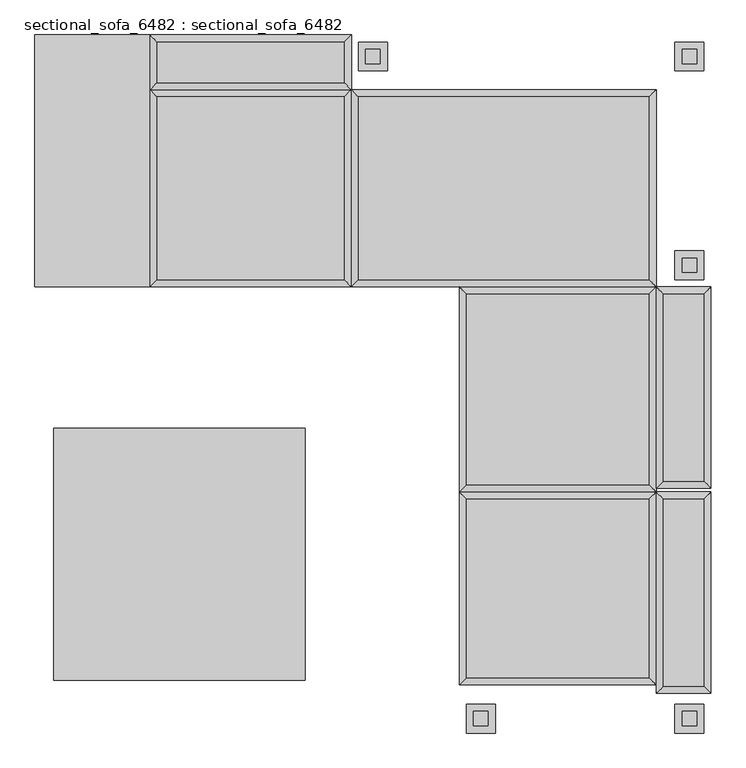
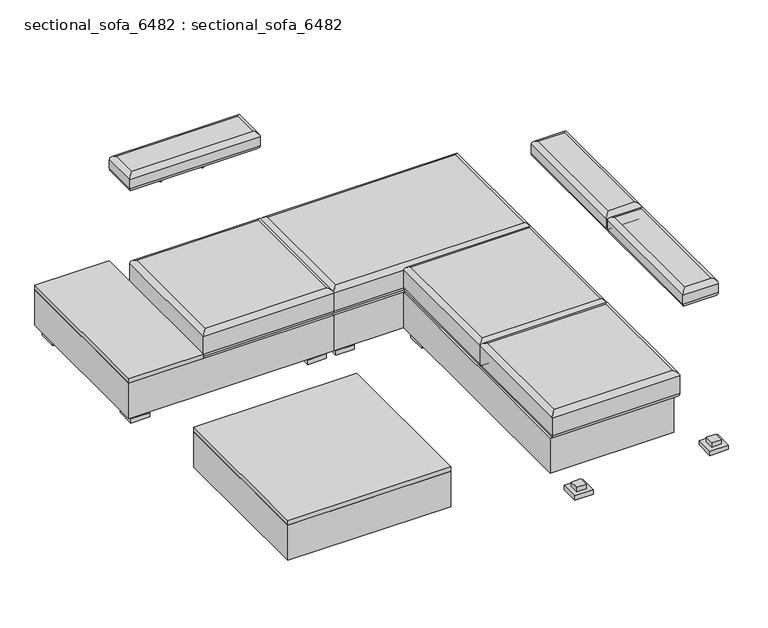
"""IFC4 building model written with IfcOpenShell, lengths in millimetres: proxy geometry, sectional_sofa_6482 : sectional_sofa_6482."""

from ifc_helpers import new_model, si_unit, point, frame, frame_2d, origin, place, context, project, spatial, polyline, circle_curve, ellipse_curve, trimmed, segment, composite_curve, outline, extrude, faceted_brep, source, transform, mapped, element, save
from ifc_brep_helpers import plane_surface, cylinder_surface, advanced_brep


def sectional_sofa_6482_sectional_sofa_6482_559db2f0(model_context):
    return source(origin(), model_context, "Body", "SolidModel", [
        extrude(outline(polyline([(-712.932438, 1291.6931081), (-712.932438, 1077.8583572), (-1.732438, 1077.8583572), (-1.732438, 402.6931081), (-1119.332438, 402.6931081), (-1119.332438, 1291.6931081), (-712.932438, 1291.6931081)])), frame((0.0, 0.0, 50.8), z_axis=(0.0, 0.0, 1.0), x_axis=(1.0, 0.0, 0.0)), (0.0, 0.0, 1.0), 203.2),
        extrude(outline(polyline([(1054.4328112, 1077.8583572), (1054.4328112, 402.6931081), (-1.732438, 402.6931081), (-1.732438, 1077.8583572), (1054.4328112, 1077.8583572)])), frame((0.0, 0.0, 50.8), z_axis=(0.0, 0.0, 1.0), x_axis=(1.0, 0.0, 0.0)), (0.0, 0.0, 1.0), 203.2),
        extrude(outline(polyline([(1054.4328112, -983.672141), (379.267562, -983.672141), (379.267562, 402.6931081), (1054.4328112, 402.6931081), (1054.4328112, -983.672141)])), frame((0.0, 0.0, 50.8), z_axis=(0.0, 0.0, 1.0), x_axis=(1.0, 0.0, 0.0)), (0.0, 0.0, 1.0), 203.2),
        faceted_brep([(-712.932438, 1291.6931081, 279.4), (-1119.332438, 1291.6931081, 279.4), (-1119.332438, 402.6931081, 279.4), (-712.932438, 402.6931081, 279.4), (-712.932438, 1098.2849958, 279.4), (-712.932438, 402.6931081, 254.0), (-1119.332438, 402.6931081, 254.0), (-1119.332438, 1291.6931081, 254.0), (-712.932438, 1291.6931081, 254.0), (-712.932438, 1098.2849958, 254.0)], [[[0, 1, 2, 3, 4]], [[5, 6, 7, 8, 9]], [[1, 0, 8, 7]], [[2, 1, 7, 6]], [[3, 2, 6, 5]], [[8, 0, 4, 3, 5, 9]]]),
        advanced_brep(
        [(404.667562, -346.6068919, 406.4), (404.667562, -977.0009907, 406.4), (1049.4594497, -977.0009907, 406.4), (1049.4594497, -346.6068919, 406.4), (404.667562, -977.0009907, 254.0), (404.667562, -346.6068919, 254.0), (1049.4594497, -346.6068919, 254.0), (1049.4594497, -977.0009907, 254.0), (1074.8594497, -321.2068919, 279.4), (1074.8594497, -321.2068919, 381.0), (1074.8594497, -1002.4009907, 381.0), (1074.8594497, -1002.4009907, 279.4), (379.267562, -321.2068919, 279.4), (379.267562, -321.2068919, 381.0), (379.267562, -1002.4009907, 279.4), (379.267562, -1002.4009907, 381.0)],
        [
            (0, 1),
            (1, 2),
            (2, 3),
            (3, 0),
            (4, 5),
            (5, 6),
            (6, 7),
            (7, 4),
            (8, 9),
            (9, 10),
            (10, 11),
            (11, 8),
            (8, 12),
            (12, 13),
            (13, 9),
            (12, 14),
            (14, 15),
            (15, 13),
            (10, 15),
            (14, 11),
            (15, 1, ellipse_curve(frame((404.667562, -977.0009907, 381.0), z_axis=(-0.7071067811865459, 0.707106781186549, 0.0), x_axis=(-0.7071067811865489, -0.7071067811865462, 0.0)), 35.9210245, 25.4)),
            (0, 13, ellipse_curve(frame((404.667562, -346.6068919, 381.0), z_axis=(-0.7071067811865489, -0.707106781186546, 0.0), x_axis=(0.707106781186546, -0.7071067811865489, 0.0)), 35.9210245, 25.4)),
            (4, 14, ellipse_curve(frame((404.667562, -977.0009907, 279.4), z_axis=(-0.7071067811865459, 0.707106781186549, 0.0), x_axis=(-0.7071067811865489, -0.7071067811865462, 0.0)), 35.9210245, 25.4)),
            (12, 5, ellipse_curve(frame((404.667562, -346.6068919, 279.4), z_axis=(-0.7071067811865489, -0.707106781186546, 0.0), x_axis=(0.707106781186546, -0.7071067811865489, 0.0)), 35.9210245, 25.4)),
            (10, 2, ellipse_curve(frame((1049.4594497, -977.0009907, 381.0), z_axis=(-0.707106781186549, -0.707106781186546, 0.0), x_axis=(0.7071067811865461, -0.7071067811865489, 0.0)), 35.9210245, 25.4)),
            (7, 11, ellipse_curve(frame((1049.4594497, -977.0009907, 279.4), z_axis=(-0.707106781186549, -0.707106781186546, 0.0), x_axis=(0.7071067811865461, -0.7071067811865489, 0.0)), 35.9210245, 25.4)),
            (9, 3, ellipse_curve(frame((1049.4594497, -346.6068919, 381.0), z_axis=(0.7071067811865461, -0.7071067811865489, 0.0), x_axis=(0.7071067811865489, 0.7071067811865461, 0.0)), 35.9210245, 25.4)),
            (6, 8, ellipse_curve(frame((1049.4594497, -346.6068919, 279.4), z_axis=(0.7071067811865461, -0.7071067811865489, 0.0), x_axis=(0.7071067811865489, 0.7071067811865461, 0.0)), 35.9210245, 25.4)),
        ],
        [
            plane_surface(frame((1074.8594497, -333.9068919, 406.4), z_axis=(0.0, 0.0, 1.0), x_axis=(0.0, 1.0, 0.0))),
            plane_surface(frame((1074.8594497, -333.9068919, 254.0), z_axis=(0.0, 0.0, -1.0), x_axis=(0.0, -1.0, 0.0))),
            plane_surface(frame((1074.8594497, -1002.4009907, 406.4), z_axis=(1.0, 0.0, 0.0), x_axis=(0.0, 0.0, -1.0))),
            plane_surface(frame((1074.8594497, -321.2068919, 406.4), z_axis=(0.0, 1.0, 0.0), x_axis=(0.0, 0.0, -1.0))),
            plane_surface(frame((379.267562, -321.2068919, 406.4), z_axis=(-1.0, 0.0, 0.0), x_axis=(0.0, 0.0, -1.0))),
            plane_surface(frame((379.267562, -1002.4009907, 406.4), z_axis=(0.0, -1.0, 0.0), x_axis=(0.0, 0.0, -1.0))),
            cylinder_surface(frame((404.667562, -321.2068919, 381.0), z_axis=(0.0, -1.0, 0.0), x_axis=(1.0, 0.0, 0.0)), 25.4),
            cylinder_surface(frame((404.667562, -321.2068919, 279.4), z_axis=(0.0, -1.0, 0.0), x_axis=(1.0, 0.0, 0.0)), 25.4),
            cylinder_surface(frame((379.267562, -977.0009907, 381.0), z_axis=(1.0, 0.0, 0.0), x_axis=(0.0, 1.0, 0.0)), 25.4),
            cylinder_surface(frame((379.267562, -977.0009907, 279.4), z_axis=(1.0, 0.0, 0.0), x_axis=(0.0, 1.0, 0.0)), 25.4),
            cylinder_surface(frame((1049.4594497, -1002.4009907, 381.0), z_axis=(0.0, 1.0, 0.0), x_axis=(-1.0, 0.0, 0.0)), 25.4),
            cylinder_surface(frame((1049.4594497, -1002.4009907, 279.4), z_axis=(0.0, 1.0, 0.0), x_axis=(-1.0, 0.0, 0.0)), 25.4),
            cylinder_surface(frame((1074.8594497, -346.6068919, 381.0), z_axis=(-1.0, 0.0, 0.0), x_axis=(0.0, -1.0, 0.0)), 25.4),
            cylinder_surface(frame((1074.8594497, -346.6068919, 279.4), z_axis=(-1.0, 0.0, 0.0), x_axis=(0.0, -1.0, 0.0)), 25.4),
        ],
        [
            (0, [[1, 2, 3, 4]]),
            (1, [[5, 6, 7, 8]]),
            (2, [[9, 10, 11, 12]]),
            (3, [[-9, 13, 14, 15]]),
            (4, [[-14, 16, 17, 18]]),
            (5, [[-11, 19, -17, 20]]),
            (6, [[21, -1, 22, -18]]),
            (7, [[23, -16, 24, -5]]),
            (8, [[-21, -19, 25, -2]]),
            (9, [[-23, -8, 26, -20]]),
            (10, [[-25, -10, 27, -3]]),
            (11, [[-26, -7, 28, -12]]),
            (12, [[-22, -4, -27, -15]]),
            (13, [[-24, -13, -28, -6]]),
        ],
    ),
        faceted_brep([(-992.332438, 1164.6931081, 25.4), (-992.332438, 1266.2931081, 25.4), (-1093.932438, 1266.2931081, 25.4), (-1093.932438, 1164.6931081, 25.4), (-1017.732438, 1240.8931081, 25.4), (-1017.732438, 1190.0931081, 25.4), (-1068.532438, 1190.0931081, 25.4), (-1068.532438, 1240.8931081, 25.4), (-992.332438, 1164.6931081, 0.0), (-1093.932438, 1164.6931081, 0.0), (-1093.932438, 1266.2931081, 0.0), (-992.332438, 1266.2931081, 0.0), (-1017.732438, 1190.0931081, 50.8), (-1017.732438, 1240.8931081, 50.8), (-1068.532438, 1240.8931081, 50.8), (-1068.532438, 1190.0931081, 50.8)], [[[0, 1, 2, 3], [4, 5, 6, 7]], [[8, 9, 10, 11]], [[1, 0, 8, 11]], [[2, 1, 11, 10]], [[3, 2, 10, 9]], [[0, 3, 9, 8]], [[12, 13, 14, 15]], [[13, 12, 5, 4]], [[14, 13, 4, 7]], [[15, 14, 7, 6]], [[12, 15, 6, 5]]]),
        faceted_brep([(-992.332438, 428.0931081, 25.4), (-992.332438, 529.6931081, 25.4), (-1093.932438, 529.6931081, 25.4), (-1093.932438, 428.0931081, 25.4), (-1017.732438, 504.2931081, 25.4), (-1017.732438, 453.4931081, 25.4), (-1068.532438, 453.4931081, 25.4), (-1068.532438, 504.2931081, 25.4), (-992.332438, 428.0931081, 0.0), (-1093.932438, 428.0931081, 0.0), (-1093.932438, 529.6931081, 0.0), (-992.332438, 529.6931081, 0.0), (-1017.732438, 453.4931081, 50.8), (-1017.732438, 504.2931081, 50.8), (-1068.532438, 504.2931081, 50.8), (-1068.532438, 453.4931081, 50.8)], [[[0, 1, 2, 3], [4, 5, 6, 7]], [[8, 9, 10, 11]], [[1, 0, 8, 11]], [[2, 1, 11, 10]], [[3, 2, 10, 9]], [[0, 3, 9, 8]], [[12, 13, 14, 15]], [[13, 12, 5, 4]], [[14, 13, 4, 7]], [[15, 14, 7, 6]], [[12, 15, 6, 5]]]),
        faceted_brep([(-27.132438, 1164.6931081, 25.4), (-27.132438, 1266.2931081, 25.4), (-128.732438, 1266.2931081, 25.4), (-128.732438, 1164.6931081, 25.4), (-52.532438, 1240.8931081, 25.4), (-52.532438, 1190.0931081, 25.4), (-103.332438, 1190.0931081, 25.4), (-103.332438, 1240.8931081, 25.4), (-27.132438, 1164.6931081, 0.0), (-128.732438, 1164.6931081, 0.0), (-128.732438, 1266.2931081, 0.0), (-27.132438, 1266.2931081, 0.0), (-52.532438, 1190.0931081, 50.8), (-52.532438, 1240.8931081, 50.8), (-103.332438, 1240.8931081, 50.8), (-103.332438, 1190.0931081, 50.8)], [[[0, 1, 2, 3], [4, 5, 6, 7]], [[8, 9, 10, 11]], [[1, 0, 8, 11]], [[2, 1, 11, 10]], [[3, 2, 10, 9]], [[0, 3, 9, 8]], [[12, 13, 14, 15]], [[13, 12, 5, 4]], [[14, 13, 4, 7]], [[15, 14, 7, 6]], [[12, 15, 6, 5]]]),
        faceted_brep([(23.667562, 1164.6931081, 25.4), (125.267562, 1164.6931081, 25.4), (125.267562, 1266.2931081, 25.4), (23.667562, 1266.2931081, 25.4), (99.867562, 1190.0931081, 25.4), (49.067562, 1190.0931081, 25.4), (49.067562, 1240.8931081, 25.4), (99.867562, 1240.8931081, 25.4), (23.667562, 1164.6931081, 0.0), (23.667562, 1266.2931081, 0.0), (125.267562, 1266.2931081, 0.0), (125.267562, 1164.6931081, 0.0), (49.067562, 1190.0931081, 50.8), (99.867562, 1190.0931081, 50.8), (99.867562, 1240.8931081, 50.8), (49.067562, 1240.8931081, 50.8)], [[[0, 1, 2, 3], [4, 5, 6, 7]], [[8, 9, 10, 11]], [[1, 0, 8, 11]], [[2, 1, 11, 10]], [[3, 2, 10, 9]], [[0, 3, 9, 8]], [[12, 13, 14, 15]], [[13, 12, 5, 4]], [[14, 13, 4, 7]], [[15, 14, 7, 6]], [[12, 15, 6, 5]]]),
        faceted_brep([(-27.132438, 428.0931081, 25.4), (-27.132438, 529.6931081, 25.4), (-128.732438, 529.6931081, 25.4), (-128.732438, 428.0931081, 25.4), (-52.532438, 504.2931081, 25.4), (-52.532438, 453.4931081, 25.4), (-103.332438, 453.4931081, 25.4), (-103.332438, 504.2931081, 25.4), (-27.132438, 428.0931081, 0.0), (-128.732438, 428.0931081, 0.0), (-128.732438, 529.6931081, 0.0), (-27.132438, 529.6931081, 0.0), (-52.532438, 453.4931081, 50.8), (-52.532438, 504.2931081, 50.8), (-103.332438, 504.2931081, 50.8), (-103.332438, 453.4931081, 50.8)], [[[0, 1, 2, 3], [4, 5, 6, 7]], [[8, 9, 10, 11]], [[1, 0, 8, 11]], [[2, 1, 11, 10]], [[3, 2, 10, 9]], [[0, 3, 9, 8]], [[12, 13, 14, 15]], [[13, 12, 5, 4]], [[14, 13, 4, 7]], [[15, 14, 7, 6]], [[12, 15, 6, 5]]]),
        faceted_brep([(23.667562, 428.0931081, 25.4), (125.267562, 428.0931081, 25.4), (125.267562, 529.6931081, 25.4), (23.667562, 529.6931081, 25.4), (99.867562, 453.4931081, 25.4), (49.067562, 453.4931081, 25.4), (49.067562, 504.2931081, 25.4), (99.867562, 504.2931081, 25.4), (23.667562, 428.0931081, 0.0), (23.667562, 529.6931081, 0.0), (125.267562, 529.6931081, 0.0), (125.267562, 428.0931081, 0.0), (49.067562, 453.4931081, 50.8), (99.867562, 453.4931081, 50.8), (99.867562, 504.2931081, 50.8), (49.067562, 504.2931081, 50.8)], [[[0, 1, 2, 3], [4, 5, 6, 7]], [[8, 9, 10, 11]], [[1, 0, 8, 11]], [[2, 1, 11, 10]], [[3, 2, 10, 9]], [[0, 3, 9, 8]], [[12, 13, 14, 15]], [[13, 12, 5, 4]], [[14, 13, 4, 7]], [[15, 14, 7, 6]], [[12, 15, 6, 5]]]),
        faceted_brep([(1242.867562, 1164.6931081, 25.4), (1242.867562, 1266.2931081, 25.4), (1141.267562, 1266.2931081, 25.4), (1141.267562, 1164.6931081, 25.4), (1217.467562, 1240.8931081, 25.4), (1217.467562, 1190.0931081, 25.4), (1166.667562, 1190.0931081, 25.4), (1166.667562, 1240.8931081, 25.4), (1242.867562, 1164.6931081, 0.0), (1141.267562, 1164.6931081, 0.0), (1141.267562, 1266.2931081, 0.0), (1242.867562, 1266.2931081, 0.0), (1217.467562, 1190.0931081, 50.8), (1217.467562, 1240.8931081, 50.8), (1166.667562, 1240.8931081, 50.8), (1166.667562, 1190.0931081, 50.8)], [[[0, 1, 2, 3], [4, 5, 6, 7]], [[8, 9, 10, 11]], [[1, 0, 8, 11]], [[2, 1, 11, 10]], [[3, 2, 10, 9]], [[0, 3, 9, 8]], [[12, 13, 14, 15]], [[13, 12, 5, 4]], [[14, 13, 4, 7]], [[15, 14, 7, 6]], [[12, 15, 6, 5]]]),
        faceted_brep([(506.267562, 377.2931081, 25.4), (404.667562, 377.2931081, 25.4), (404.667562, 275.6931081, 25.4), (506.267562, 275.6931081, 25.4), (430.067562, 351.8931081, 25.4), (480.867562, 351.8931081, 25.4), (480.867562, 301.0931081, 25.4), (430.067562, 301.0931081, 25.4), (506.267562, 377.2931081, 0.0), (506.267562, 275.6931081, 0.0), (404.667562, 275.6931081, 0.0), (404.667562, 377.2931081, 0.0), (480.867562, 351.8931081, 50.8), (430.067562, 351.8931081, 50.8), (430.067562, 301.0931081, 50.8), (480.867562, 301.0931081, 50.8)], [[[0, 1, 2, 3], [4, 5, 6, 7]], [[8, 9, 10, 11]], [[1, 0, 8, 11]], [[2, 1, 11, 10]], [[3, 2, 10, 9]], [[0, 3, 9, 8]], [[12, 13, 14, 15]], [[13, 12, 5, 4]], [[14, 13, 4, 7]], [[15, 14, 7, 6]], [[12, 15, 6, 5]]]),
        faceted_brep([(1242.867562, 428.0931081, 25.4), (1242.867562, 529.6931081, 25.4), (1141.267562, 529.6931081, 25.4), (1141.267562, 428.0931081, 25.4), (1217.467562, 504.2931081, 25.4), (1217.467562, 453.4931081, 25.4), (1166.667562, 453.4931081, 25.4), (1166.667562, 504.2931081, 25.4), (1242.867562, 428.0931081, 0.0), (1141.267562, 428.0931081, 0.0), (1141.267562, 529.6931081, 0.0), (1242.867562, 529.6931081, 0.0), (1217.467562, 453.4931081, 50.8), (1217.467562, 504.2931081, 50.8), (1166.667562, 504.2931081, 50.8), (1166.667562, 453.4931081, 50.8)], [[[0, 1, 2, 3], [4, 5, 6, 7]], [[8, 9, 10, 11]], [[1, 0, 8, 11]], [[2, 1, 11, 10]], [[3, 2, 10, 9]], [[0, 3, 9, 8]], [[12, 13, 14, 15]], [[13, 12, 5, 4]], [[14, 13, 4, 7]], [[15, 14, 7, 6]], [[12, 15, 6, 5]]]),
        faceted_brep([(1242.867562, 377.2931081, 25.4), (1141.267562, 377.2931081, 25.4), (1141.267562, 275.6931081, 25.4), (1242.867562, 275.6931081, 25.4), (1166.667562, 351.8931081, 25.4), (1217.467562, 351.8931081, 25.4), (1217.467562, 301.0931081, 25.4), (1166.667562, 301.0931081, 25.4), (1242.867562, 377.2931081, 0.0), (1242.867562, 275.6931081, 0.0), (1141.267562, 275.6931081, 0.0), (1141.267562, 377.2931081, 0.0), (1217.467562, 351.8931081, 50.8), (1166.667562, 351.8931081, 50.8), (1166.667562, 301.0931081, 50.8), (1217.467562, 301.0931081, 50.8)], [[[0, 1, 2, 3], [4, 5, 6, 7]], [[8, 9, 10, 11]], [[1, 0, 8, 11]], [[2, 1, 11, 10]], [[3, 2, 10, 9]], [[0, 3, 9, 8]], [[12, 13, 14, 15]], [[13, 12, 5, 4]], [[14, 13, 4, 7]], [[15, 14, 7, 6]], [[12, 15, 6, 5]]]),
        faceted_brep([(506.267562, -1172.1068919, 25.4), (506.267562, -1070.5068919, 25.4), (404.667562, -1070.5068919, 25.4), (404.667562, -1172.1068919, 25.4), (480.867562, -1095.9068919, 25.4), (480.867562, -1146.7068919, 25.4), (430.067562, -1146.7068919, 25.4), (430.067562, -1095.9068919, 25.4), (506.267562, -1172.1068919, 0.0), (404.667562, -1172.1068919, 0.0), (404.667562, -1070.5068919, 0.0), (506.267562, -1070.5068919, 0.0), (480.867562, -1146.7068919, 50.8), (480.867562, -1095.9068919, 50.8), (430.067562, -1095.9068919, 50.8), (430.067562, -1146.7068919, 50.8)], [[[0, 1, 2, 3], [4, 5, 6, 7]], [[8, 9, 10, 11]], [[1, 0, 8, 11]], [[2, 1, 11, 10]], [[3, 2, 10, 9]], [[0, 3, 9, 8]], [[12, 13, 14, 15]], [[13, 12, 5, 4]], [[14, 13, 4, 7]], [[15, 14, 7, 6]], [[12, 15, 6, 5]]]),
        faceted_brep([(1242.867562, -1172.1068919, 25.4), (1242.867562, -1070.5068919, 25.4), (1141.267562, -1070.5068919, 25.4), (1141.267562, -1172.1068919, 25.4), (1217.467562, -1095.9068919, 25.4), (1217.467562, -1146.7068919, 25.4), (1166.667562, -1146.7068919, 25.4), (1166.667562, -1095.9068919, 25.4), (1242.867562, -1172.1068919, 0.0), (1141.267562, -1172.1068919, 0.0), (1141.267562, -1070.5068919, 0.0), (1242.867562, -1070.5068919, 0.0), (1217.467562, -1146.7068919, 50.8), (1217.467562, -1095.9068919, 50.8), (1166.667562, -1095.9068919, 50.8), (1166.667562, -1146.7068919, 50.8)], [[[0, 1, 2, 3], [4, 5, 6, 7]], [[8, 9, 10, 11]], [[1, 0, 8, 11]], [[2, 1, 11, 10]], [[3, 2, 10, 9]], [[0, 3, 9, 8]], [[12, 13, 14, 15]], [[13, 12, 5, 4]], [[14, 13, 4, 7]], [[15, 14, 7, 6]], [[12, 15, 6, 5]]]),
        extrude(outline(composite_curve([segment(trimmed(circle_curve(frame_2d((-482.8859111, 1206.7842798)), 6.35), [point((-489.2359111, 1206.7842798))], [point((-476.5359111, 1206.7842798))], False, "CARTESIAN"), True, "CONTINUOUS"), segment(trimmed(circle_curve(frame_2d((-482.8859111, 1206.7842798)), 6.35), [point((-476.5359111, 1206.7842798))], [point((-489.2359111, 1206.7842798))], False, "CARTESIAN"), True, "CONTINUOUS")], self_intersect=False)), frame((0.0, 0.0, 711.2), z_axis=(0.0, 0.0, 1.0), x_axis=(1.0, 0.0, 0.0)), (0.0, 0.0, 1.0), 76.2),
        extrude(outline(composite_curve([segment(trimmed(circle_curve(frame_2d((-254.2859111, 1206.7842798)), 6.35), [point((-260.6359111, 1206.7842798))], [point((-247.9359111, 1206.7842798))], False, "CARTESIAN"), True, "CONTINUOUS"), segment(trimmed(circle_curve(frame_2d((-254.2859111, 1206.7842798)), 6.35), [point((-247.9359111, 1206.7842798))], [point((-260.6359111, 1206.7842798))], False, "CARTESIAN"), True, "CONTINUOUS")], self_intersect=False)), frame((0.0, 0.0, 711.2), z_axis=(0.0, 0.0, 1.0), x_axis=(1.0, 0.0, 0.0)), (0.0, 0.0, 1.0), 76.2),
        extrude(outline(composite_curve([segment(trimmed(circle_curve(frame_2d((1173.6454882, 148.0415505)), 6.35), [point((1173.6454882, 154.3915505))], [point((1173.6454882, 141.6915505))], False, "CARTESIAN"), True, "CONTINUOUS"), segment(trimmed(circle_curve(frame_2d((1173.6454882, 148.0415505)), 6.35), [point((1173.6454882, 141.6915505))], [point((1173.6454882, 154.3915505))], False, "CARTESIAN"), True, "CONTINUOUS")], self_intersect=False)), frame((0.0, 0.0, 711.2), z_axis=(0.0, 0.0, 1.0), x_axis=(1.0, 0.0, 0.0)), (0.0, 0.0, 1.0), 76.2),
        extrude(outline(composite_curve([segment(trimmed(circle_curve(frame_2d((1173.6454882, -80.5584495)), 6.35), [point((1173.6454882, -74.2084495))], [point((1173.6454882, -86.9084495))], False, "CARTESIAN"), True, "CONTINUOUS"), segment(trimmed(circle_curve(frame_2d((1173.6454882, -80.5584495)), 6.35), [point((1173.6454882, -86.9084495))], [point((1173.6454882, -74.2084495))], False, "CARTESIAN"), True, "CONTINUOUS")], self_intersect=False)), frame((0.0, 0.0, 711.2), z_axis=(0.0, 0.0, 1.0), x_axis=(1.0, 0.0, 0.0)), (0.0, 0.0, 1.0), 76.2),
        extrude(outline(composite_curve([segment(trimmed(circle_curve(frame_2d((1173.6454882, -563.1584495)), 6.35), [point((1173.6454882, -556.8084495))], [point((1173.6454882, -569.5084495))], False, "CARTESIAN"), True, "CONTINUOUS"), segment(trimmed(circle_curve(frame_2d((1173.6454882, -563.1584495)), 6.35), [point((1173.6454882, -569.5084495))], [point((1173.6454882, -556.8084495))], False, "CARTESIAN"), True, "CONTINUOUS")], self_intersect=False)), frame((0.0, 0.0, 711.2), z_axis=(0.0, 0.0, 1.0), x_axis=(1.0, 0.0, 0.0)), (0.0, 0.0, 1.0), 76.2),
        extrude(outline(composite_curve([segment(trimmed(circle_curve(frame_2d((1173.6454882, -791.7584495)), 6.35), [point((1173.6454882, -785.4084495))], [point((1173.6454882, -798.1084495))], False, "CARTESIAN"), True, "CONTINUOUS"), segment(trimmed(circle_curve(frame_2d((1173.6454882, -791.7584495)), 6.35), [point((1173.6454882, -798.1084495))], [point((1173.6454882, -785.4084495))], False, "CARTESIAN"), True, "CONTINUOUS")], self_intersect=False)), frame((0.0, 0.0, 711.2), z_axis=(0.0, 0.0, 1.0), x_axis=(1.0, 0.0, 0.0)), (0.0, 0.0, 1.0), 76.2),
        advanced_brep(
        [(-687.532438, 1123.6849958, 889.0), (-27.132438, 1123.6849958, 889.0), (-27.132438, 1266.2931081, 889.0), (-687.532438, 1266.2931081, 889.0), (-27.132438, 1123.6849958, 787.4), (-687.532438, 1123.6849958, 787.4), (-687.532438, 1266.2931081, 787.4), (-27.132438, 1266.2931081, 787.4), (-1.732438, 1291.6931081, 863.6), (-1.732438, 1291.6931081, 812.8), (-712.932438, 1291.6931081, 812.8), (-712.932438, 1291.6931081, 863.6), (-712.932438, 1098.2849958, 812.8), (-712.932438, 1098.2849958, 863.6), (-1.732438, 1098.2849958, 812.8), (-1.732438, 1098.2849958, 863.6)],
        [
            (0, 1),
            (1, 2),
            (2, 3),
            (3, 0),
            (4, 5),
            (5, 6),
            (6, 7),
            (7, 4),
            (8, 9),
            (9, 10),
            (10, 11),
            (11, 8),
            (10, 12),
            (12, 13),
            (13, 11),
            (12, 14),
            (14, 15),
            (15, 13),
            (8, 15),
            (14, 9),
            (15, 1, ellipse_curve(frame((-27.132438, 1123.6849958, 863.6), z_axis=(-0.7071067811865475, -0.7071067811865475, 0.0), x_axis=(0.7071067811865476, -0.7071067811865474, 0.0)), 35.9210245, 25.4)),
            (0, 13, ellipse_curve(frame((-687.532438, 1123.6849958, 863.6), z_axis=(0.7071067811865475, -0.7071067811865475, 0.0), x_axis=(0.7071067811865476, 0.7071067811865474, 0.0)), 35.9210245, 25.4)),
            (4, 14, ellipse_curve(frame((-27.132438, 1123.6849958, 812.8), z_axis=(-0.7071067811865475, -0.7071067811865475, 0.0), x_axis=(0.7071067811865476, -0.7071067811865474, 0.0)), 35.9210245, 25.4)),
            (12, 5, ellipse_curve(frame((-687.532438, 1123.6849958, 812.8), z_axis=(0.7071067811865475, -0.7071067811865475, 0.0), x_axis=(0.7071067811865476, 0.7071067811865474, 0.0)), 35.9210245, 25.4)),
            (8, 2, ellipse_curve(frame((-27.132438, 1266.2931081, 863.6), z_axis=(0.7071067811865475, -0.7071067811865475, 0.0), x_axis=(0.7071067811865474, 0.7071067811865476, 0.0)), 35.9210245, 25.4)),
            (7, 9, ellipse_curve(frame((-27.132438, 1266.2931081, 812.8), z_axis=(0.7071067811865475, -0.7071067811865475, 0.0), x_axis=(0.7071067811865474, 0.7071067811865476, 0.0)), 35.9210245, 25.4)),
            (11, 3, ellipse_curve(frame((-687.532438, 1266.2931081, 863.6), z_axis=(0.7071067811865475, 0.7071067811865475, 0.0), x_axis=(-0.7071067811865476, 0.7071067811865474, 0.0)), 35.9210245, 25.4)),
            (6, 10, ellipse_curve(frame((-687.532438, 1266.2931081, 812.8), z_axis=(0.7071067811865475, 0.7071067811865475, 0.0), x_axis=(-0.7071067811865476, 0.7071067811865474, 0.0)), 35.9210245, 25.4)),
        ],
        [
            plane_surface(frame((-712.932438, 1291.6931081, 889.0), z_axis=(0.0, 0.0, 1.0), x_axis=(-1.0, 0.0, 0.0))),
            plane_surface(frame((-712.932438, 1291.6931081, 787.4), z_axis=(0.0, 0.0, -1.0), x_axis=(1.0, 0.0, 0.0))),
            plane_surface(frame((-1.732438, 1291.6931081, 889.0), z_axis=(0.0, 1.0, 0.0), x_axis=(0.0, 0.0, -1.0))),
            plane_surface(frame((-712.932438, 1291.6931081, 889.0), z_axis=(-1.0, 0.0, 0.0), x_axis=(0.0, 0.0, -1.0))),
            plane_surface(frame((-712.932438, 1098.2849958, 889.0), z_axis=(0.0, -1.0, 0.0), x_axis=(0.0, 0.0, -1.0))),
            plane_surface(frame((-1.732438, 1098.2849958, 889.0), z_axis=(1.0, 0.0, 0.0), x_axis=(0.0, 0.0, -1.0))),
            cylinder_surface(frame((-712.932438, 1123.6849958, 863.6), z_axis=(1.0, 0.0, 0.0), x_axis=(0.0, 1.0, 0.0)), 25.4),
            cylinder_surface(frame((-712.932438, 1123.6849958, 812.8), z_axis=(1.0, 0.0, 0.0), x_axis=(0.0, 1.0, 0.0)), 25.4),
            cylinder_surface(frame((-27.132438, 1098.2849958, 863.6), z_axis=(0.0, 1.0, 0.0), x_axis=(-1.0, 0.0, 0.0)), 25.4),
            cylinder_surface(frame((-27.132438, 1098.2849958, 812.8), z_axis=(0.0, 1.0, 0.0), x_axis=(-1.0, 0.0, 0.0)), 25.4),
            cylinder_surface(frame((-1.732438, 1266.2931081, 863.6), z_axis=(-1.0, 0.0, 0.0), x_axis=(0.0, -1.0, 0.0)), 25.4),
            cylinder_surface(frame((-1.732438, 1266.2931081, 812.8), z_axis=(-1.0, 0.0, 0.0), x_axis=(0.0, -1.0, 0.0)), 25.4),
            cylinder_surface(frame((-687.532438, 1291.6931081, 863.6), z_axis=(0.0, -1.0, 0.0), x_axis=(1.0, 0.0, 0.0)), 25.4),
            cylinder_surface(frame((-687.532438, 1291.6931081, 812.8), z_axis=(0.0, -1.0, 0.0), x_axis=(1.0, 0.0, 0.0)), 25.4),
        ],
        [
            (0, [[1, 2, 3, 4]]),
            (1, [[5, 6, 7, 8]]),
            (2, [[9, 10, 11, 12]]),
            (3, [[-11, 13, 14, 15]]),
            (4, [[-14, 16, 17, 18]]),
            (5, [[-9, 19, -17, 20]]),
            (6, [[21, -1, 22, -18]]),
            (7, [[23, -16, 24, -5]]),
            (8, [[-21, -19, 25, -2]]),
            (9, [[-23, -8, 26, -20]]),
            (10, [[-25, -12, 27, -3]]),
            (11, [[-26, -7, 28, -10]]),
            (12, [[-22, -4, -27, -15]]),
            (13, [[-24, -13, -28, -6]]),
        ],
    ),
        advanced_brep(
        [(1100.2594497, 377.2931081, 889.0), (1100.2594497, -283.1068919, 889.0), (1242.867562, -283.1068919, 889.0), (1242.867562, 377.2931081, 889.0), (1100.2594497, -283.1068919, 787.4), (1100.2594497, 377.2931081, 787.4), (1242.867562, 377.2931081, 787.4), (1242.867562, -283.1068919, 787.4), (1268.267562, -308.5068919, 863.6), (1268.267562, -308.5068919, 812.8), (1268.267562, 402.6931081, 812.8), (1268.267562, 402.6931081, 863.6), (1074.8594497, 402.6931081, 812.8), (1074.8594497, 402.6931081, 863.6), (1074.8594497, -308.5068919, 812.8), (1074.8594497, -308.5068919, 863.6)],
        [
            (0, 1),
            (1, 2),
            (2, 3),
            (3, 0),
            (4, 5),
            (5, 6),
            (6, 7),
            (7, 4),
            (8, 9),
            (9, 10),
            (10, 11),
            (11, 8),
            (10, 12),
            (12, 13),
            (13, 11),
            (12, 14),
            (14, 15),
            (15, 13),
            (8, 15),
            (14, 9),
            (15, 1, ellipse_curve(frame((1100.2594497, -283.1068919, 863.6), z_axis=(-0.7071067811865487, 0.7071067811865462, 0.0), x_axis=(-0.7071067811865462, -0.7071067811865488, 0.0)), 35.9210245, 25.4)),
            (0, 13, ellipse_curve(frame((1100.2594497, 377.2931081, 863.6), z_axis=(-0.7071067811865461, -0.7071067811865489, 0.0), x_axis=(0.7071067811865489, -0.7071067811865461, 0.0)), 35.9210245, 25.4)),
            (4, 14, ellipse_curve(frame((1100.2594497, -283.1068919, 812.8), z_axis=(-0.7071067811865487, 0.7071067811865462, 0.0), x_axis=(-0.7071067811865462, -0.7071067811865488, 0.0)), 35.9210245, 25.4)),
            (12, 5, ellipse_curve(frame((1100.2594497, 377.2931081, 812.8), z_axis=(-0.7071067811865461, -0.7071067811865489, 0.0), x_axis=(0.7071067811865489, -0.7071067811865461, 0.0)), 35.9210245, 25.4)),
            (8, 2, ellipse_curve(frame((1242.867562, -283.1068919, 863.6), z_axis=(-0.7071067811865462, -0.7071067811865489, 0.0), x_axis=(0.7071067811865487, -0.7071067811865464, 0.0)), 35.9210245, 25.4)),
            (7, 9, ellipse_curve(frame((1242.867562, -283.1068919, 812.8), z_axis=(-0.7071067811865462, -0.7071067811865489, 0.0), x_axis=(0.7071067811865487, -0.7071067811865464, 0.0)), 35.9210245, 25.4)),
            (11, 3, ellipse_curve(frame((1242.867562, 377.2931081, 863.6), z_axis=(0.707106781186549, -0.707106781186546, 0.0), x_axis=(0.707106781186546, 0.707106781186549, 0.0)), 35.9210245, 25.4)),
            (6, 10, ellipse_curve(frame((1242.867562, 377.2931081, 812.8), z_axis=(0.707106781186549, -0.707106781186546, 0.0), x_axis=(0.707106781186546, 0.707106781186549, 0.0)), 35.9210245, 25.4)),
        ],
        [
            plane_surface(frame((1268.267562, 402.6931081, 889.0), z_axis=(0.0, 0.0, 1.0), x_axis=(0.0, 1.0, 0.0))),
            plane_surface(frame((1268.267562, 402.6931081, 787.4), z_axis=(0.0, 0.0, -1.0), x_axis=(0.0, -1.0, 0.0))),
            plane_surface(frame((1268.267562, -308.5068919, 889.0), z_axis=(1.0, 0.0, 0.0), x_axis=(0.0, 0.0, -1.0))),
            plane_surface(frame((1268.267562, 402.6931081, 889.0), z_axis=(0.0, 1.0, 0.0), x_axis=(0.0, 0.0, -1.0))),
            plane_surface(frame((1074.8594497, 402.6931081, 889.0), z_axis=(-1.0, 0.0, 0.0), x_axis=(0.0, 0.0, -1.0))),
            plane_surface(frame((1074.8594497, -308.5068919, 889.0), z_axis=(0.0, -1.0, 0.0), x_axis=(0.0, 0.0, -1.0))),
            cylinder_surface(frame((1100.2594497, 402.6931081, 863.6), z_axis=(0.0, -1.0, 0.0), x_axis=(1.0, 0.0, 0.0)), 25.4),
            cylinder_surface(frame((1100.2594497, 402.6931081, 812.8), z_axis=(0.0, -1.0, 0.0), x_axis=(1.0, 0.0, 0.0)), 25.4),
            cylinder_surface(frame((1074.8594497, -283.1068919, 863.6), z_axis=(1.0, 0.0, 0.0), x_axis=(0.0, 1.0, 0.0)), 25.4),
            cylinder_surface(frame((1074.8594497, -283.1068919, 812.8), z_axis=(1.0, 0.0, 0.0), x_axis=(0.0, 1.0, 0.0)), 25.4),
            cylinder_surface(frame((1242.867562, -308.5068919, 863.6), z_axis=(0.0, 1.0, 0.0), x_axis=(-1.0, 0.0, 0.0)), 25.4),
            cylinder_surface(frame((1242.867562, -308.5068919, 812.8), z_axis=(0.0, 1.0, 0.0), x_axis=(-1.0, 0.0, 0.0)), 25.4),
            cylinder_surface(frame((1268.267562, 377.2931081, 863.6), z_axis=(-1.0, 0.0, 0.0), x_axis=(0.0, -1.0, 0.0)), 25.4),
            cylinder_surface(frame((1268.267562, 377.2931081, 812.8), z_axis=(-1.0, 0.0, 0.0), x_axis=(0.0, -1.0, 0.0)), 25.4),
        ],
        [
            (0, [[1, 2, 3, 4]]),
            (1, [[5, 6, 7, 8]]),
            (2, [[9, 10, 11, 12]]),
            (3, [[-11, 13, 14, 15]]),
            (4, [[-14, 16, 17, 18]]),
            (5, [[-9, 19, -17, 20]]),
            (6, [[21, -1, 22, -18]]),
            (7, [[23, -16, 24, -5]]),
            (8, [[-21, -19, 25, -2]]),
            (9, [[-23, -8, 26, -20]]),
            (10, [[-25, -12, 27, -3]]),
            (11, [[-26, -7, 28, -10]]),
            (12, [[-22, -4, -27, -15]]),
            (13, [[-24, -13, -28, -6]]),
        ],
    ),
        advanced_brep(
        [(1100.2594497, -346.6068919, 889.0), (1100.2594497, -1007.0068919, 889.0), (1242.867562, -1007.0068919, 889.0), (1242.867562, -346.6068919, 889.0), (1100.2594497, -1007.0068919, 787.4), (1100.2594497, -346.6068919, 787.4), (1242.867562, -346.6068919, 787.4), (1242.867562, -1007.0068919, 787.4), (1268.267562, -1032.4068919, 863.6), (1268.267562, -1032.4068919, 812.8), (1268.267562, -321.2068919, 812.8), (1268.267562, -321.2068919, 863.6), (1074.8594497, -321.2068919, 812.8), (1074.8594497, -321.2068919, 863.6), (1074.8594497, -1032.4068919, 812.8), (1074.8594497, -1032.4068919, 863.6)],
        [
            (0, 1),
            (1, 2),
            (2, 3),
            (3, 0),
            (4, 5),
            (5, 6),
            (6, 7),
            (7, 4),
            (8, 9),
            (9, 10),
            (10, 11),
            (11, 8),
            (10, 12),
            (12, 13),
            (13, 11),
            (12, 14),
            (14, 15),
            (15, 13),
            (8, 15),
            (14, 9),
            (15, 1, ellipse_curve(frame((1100.2594497, -1007.0068919, 863.6), z_axis=(-0.7071067811865491, 0.7071067811865459, 0.0), x_axis=(-0.7071067811865458, -0.7071067811865491, 0.0)), 35.9210245, 25.4)),
            (0, 13, ellipse_curve(frame((1100.2594497, -346.6068919, 863.6), z_axis=(-0.7071067811865461, -0.7071067811865489, 0.0), x_axis=(0.7071067811865489, -0.707106781186546, 0.0)), 35.9210245, 25.4)),
            (4, 14, ellipse_curve(frame((1100.2594497, -1007.0068919, 812.8), z_axis=(-0.7071067811865491, 0.7071067811865459, 0.0), x_axis=(-0.7071067811865458, -0.7071067811865491, 0.0)), 35.9210245, 25.4)),
            (12, 5, ellipse_curve(frame((1100.2594497, -346.6068919, 812.8), z_axis=(-0.7071067811865461, -0.7071067811865489, 0.0), x_axis=(0.7071067811865489, -0.707106781186546, 0.0)), 35.9210245, 25.4)),
            (8, 2, ellipse_curve(frame((1242.867562, -1007.0068919, 863.6), z_axis=(-0.7071067811865459, -0.7071067811865491, 0.0), x_axis=(0.7071067811865491, -0.7071067811865458, 0.0)), 35.9210245, 25.4)),
            (7, 9, ellipse_curve(frame((1242.867562, -1007.0068919, 812.8), z_axis=(-0.7071067811865459, -0.7071067811865491, 0.0), x_axis=(0.7071067811865491, -0.7071067811865458, 0.0)), 35.9210245, 25.4)),
            (11, 3, ellipse_curve(frame((1242.867562, -346.6068919, 863.6), z_axis=(0.7071067811865489, -0.707106781186546, 0.0), x_axis=(0.7071067811865459, 0.7071067811865491, 0.0)), 35.9210245, 25.4)),
            (6, 10, ellipse_curve(frame((1242.867562, -346.6068919, 812.8), z_axis=(0.7071067811865489, -0.707106781186546, 0.0), x_axis=(0.7071067811865459, 0.7071067811865491, 0.0)), 35.9210245, 25.4)),
        ],
        [
            plane_surface(frame((1268.267562, -321.2068919, 889.0), z_axis=(0.0, 0.0, 1.0), x_axis=(0.0, 1.0, 0.0))),
            plane_surface(frame((1268.267562, -321.2068919, 787.4), z_axis=(0.0, 0.0, -1.0), x_axis=(0.0, -1.0, 0.0))),
            plane_surface(frame((1268.267562, -1032.4068919, 889.0), z_axis=(1.0, 0.0, 0.0), x_axis=(0.0, 0.0, -1.0))),
            plane_surface(frame((1268.267562, -321.2068919, 889.0), z_axis=(0.0, 1.0, 0.0), x_axis=(0.0, 0.0, -1.0))),
            plane_surface(frame((1074.8594497, -321.2068919, 889.0), z_axis=(-1.0, 0.0, 0.0), x_axis=(0.0, 0.0, -1.0))),
            plane_surface(frame((1074.8594497, -1032.4068919, 889.0), z_axis=(0.0, -1.0, 0.0), x_axis=(0.0, 0.0, -1.0))),
            cylinder_surface(frame((1100.2594497, -321.2068919, 863.6), z_axis=(0.0, -1.0, 0.0), x_axis=(1.0, 0.0, 0.0)), 25.4),
            cylinder_surface(frame((1100.2594497, -321.2068919, 812.8), z_axis=(0.0, -1.0, 0.0), x_axis=(1.0, 0.0, 0.0)), 25.4),
            cylinder_surface(frame((1074.8594497, -1007.0068919, 863.6), z_axis=(1.0, 0.0, 0.0), x_axis=(0.0, 1.0, 0.0)), 25.4),
            cylinder_surface(frame((1074.8594497, -1007.0068919, 812.8), z_axis=(1.0, 0.0, 0.0), x_axis=(0.0, 1.0, 0.0)), 25.4),
            cylinder_surface(frame((1242.867562, -1032.4068919, 863.6), z_axis=(0.0, 1.0, 0.0), x_axis=(-1.0, 0.0, 0.0)), 25.4),
            cylinder_surface(frame((1242.867562, -1032.4068919, 812.8), z_axis=(0.0, 1.0, 0.0), x_axis=(-1.0, 0.0, 0.0)), 25.4),
            cylinder_surface(frame((1268.267562, -346.6068919, 863.6), z_axis=(-1.0, 0.0, 0.0), x_axis=(0.0, -1.0, 0.0)), 25.4),
            cylinder_surface(frame((1268.267562, -346.6068919, 812.8), z_axis=(-1.0, 0.0, 0.0), x_axis=(0.0, -1.0, 0.0)), 25.4),
        ],
        [
            (0, [[1, 2, 3, 4]]),
            (1, [[5, 6, 7, 8]]),
            (2, [[9, 10, 11, 12]]),
            (3, [[-11, 13, 14, 15]]),
            (4, [[-14, 16, 17, 18]]),
            (5, [[-9, 19, -17, 20]]),
            (6, [[21, -1, 22, -18]]),
            (7, [[23, -16, 24, -5]]),
            (8, [[-21, -19, 25, -2]]),
            (9, [[-23, -8, 26, -20]]),
            (10, [[-25, -12, 27, -3]]),
            (11, [[-26, -7, 28, -10]]),
            (12, [[-22, -4, -27, -15]]),
            (13, [[-24, -13, -28, -6]]),
        ],
    ),
        advanced_brep(
        [(-687.532438, 428.0931081, 406.4), (-27.132438, 428.0931081, 406.4), (-27.132438, 1072.8849958, 406.4), (-687.532438, 1072.8849958, 406.4), (-27.132438, 428.0931081, 254.0), (-687.532438, 428.0931081, 254.0), (-687.532438, 1072.8849958, 254.0), (-27.132438, 1072.8849958, 254.0), (-1.732438, 1098.2849958, 381.0), (-1.732438, 1098.2849958, 279.4), (-712.932438, 1098.2849958, 279.4), (-712.932438, 1098.2849958, 381.0), (-712.932438, 402.6931081, 279.4), (-712.932438, 402.6931081, 381.0), (-1.732438, 402.6931081, 279.4), (-1.732438, 402.6931081, 381.0)],
        [
            (0, 1),
            (1, 2),
            (2, 3),
            (3, 0),
            (4, 5),
            (5, 6),
            (6, 7),
            (7, 4),
            (8, 9),
            (9, 10),
            (10, 11),
            (11, 8),
            (10, 12),
            (12, 13),
            (13, 11),
            (12, 14),
            (14, 15),
            (15, 13),
            (8, 15),
            (14, 9),
            (15, 1, ellipse_curve(frame((-27.132438, 428.0931081, 381.0), z_axis=(-0.7071067811865475, -0.7071067811865475, 0.0), x_axis=(0.7071067811865476, -0.7071067811865474, 0.0)), 35.9210245, 25.4)),
            (0, 13, ellipse_curve(frame((-687.532438, 428.0931081, 381.0), z_axis=(0.7071067811865475, -0.7071067811865475, 0.0), x_axis=(0.7071067811865476, 0.7071067811865474, 0.0)), 35.9210245, 25.4)),
            (4, 14, ellipse_curve(frame((-27.132438, 428.0931081, 279.4), z_axis=(-0.7071067811865475, -0.7071067811865475, 0.0), x_axis=(0.7071067811865476, -0.7071067811865474, 0.0)), 35.9210245, 25.4)),
            (12, 5, ellipse_curve(frame((-687.532438, 428.0931081, 279.4), z_axis=(0.7071067811865475, -0.7071067811865475, 0.0), x_axis=(0.7071067811865476, 0.7071067811865474, 0.0)), 35.9210245, 25.4)),
            (8, 2, ellipse_curve(frame((-27.132438, 1072.8849958, 381.0), z_axis=(0.7071067811865475, -0.7071067811865475, 0.0), x_axis=(0.7071067811865474, 0.7071067811865476, 0.0)), 35.9210245, 25.4)),
            (7, 9, ellipse_curve(frame((-27.132438, 1072.8849958, 279.4), z_axis=(0.7071067811865475, -0.7071067811865475, 0.0), x_axis=(0.7071067811865474, 0.7071067811865476, 0.0)), 35.9210245, 25.4)),
            (11, 3, ellipse_curve(frame((-687.532438, 1072.8849958, 381.0), z_axis=(0.7071067811865475, 0.7071067811865475, 0.0), x_axis=(-0.7071067811865476, 0.7071067811865474, 0.0)), 35.9210245, 25.4)),
            (6, 10, ellipse_curve(frame((-687.532438, 1072.8849958, 279.4), z_axis=(0.7071067811865475, 0.7071067811865475, 0.0), x_axis=(-0.7071067811865476, 0.7071067811865474, 0.0)), 35.9210245, 25.4)),
        ],
        [
            plane_surface(frame((-712.932438, 1098.2849958, 406.4), z_axis=(0.0, 0.0, 1.0), x_axis=(-1.0, 0.0, 0.0))),
            plane_surface(frame((-712.932438, 1098.2849958, 254.0), z_axis=(0.0, 0.0, -1.0), x_axis=(1.0, 0.0, 0.0))),
            plane_surface(frame((-1.732438, 1098.2849958, 406.4), z_axis=(0.0, 1.0, 0.0), x_axis=(0.0, 0.0, -1.0))),
            plane_surface(frame((-712.932438, 1098.2849958, 406.4), z_axis=(-1.0, 0.0, 0.0), x_axis=(0.0, 0.0, -1.0))),
            plane_surface(frame((-712.932438, 402.6931081, 406.4), z_axis=(0.0, -1.0, 0.0), x_axis=(0.0, 0.0, -1.0))),
            plane_surface(frame((-1.732438, 402.6931081, 406.4), z_axis=(1.0, 0.0, 0.0), x_axis=(0.0, 0.0, -1.0))),
            cylinder_surface(frame((-712.932438, 428.0931081, 381.0), z_axis=(1.0, 0.0, 0.0), x_axis=(0.0, 1.0, 0.0)), 25.4),
            cylinder_surface(frame((-712.932438, 428.0931081, 279.4), z_axis=(1.0, 0.0, 0.0), x_axis=(0.0, 1.0, 0.0)), 25.4),
            cylinder_surface(frame((-27.132438, 402.6931081, 381.0), z_axis=(0.0, 1.0, 0.0), x_axis=(-1.0, 0.0, 0.0)), 25.4),
            cylinder_surface(frame((-27.132438, 402.6931081, 279.4), z_axis=(0.0, 1.0, 0.0), x_axis=(-1.0, 0.0, 0.0)), 25.4),
            cylinder_surface(frame((-1.732438, 1072.8849958, 381.0), z_axis=(-1.0, 0.0, 0.0), x_axis=(0.0, -1.0, 0.0)), 25.4),
            cylinder_surface(frame((-1.732438, 1072.8849958, 279.4), z_axis=(-1.0, 0.0, 0.0), x_axis=(0.0, -1.0, 0.0)), 25.4),
            cylinder_surface(frame((-687.532438, 1098.2849958, 381.0), z_axis=(0.0, -1.0, 0.0), x_axis=(1.0, 0.0, 0.0)), 25.4),
            cylinder_surface(frame((-687.532438, 1098.2849958, 279.4), z_axis=(0.0, -1.0, 0.0), x_axis=(1.0, 0.0, 0.0)), 25.4),
        ],
        [
            (0, [[1, 2, 3, 4]]),
            (1, [[5, 6, 7, 8]]),
            (2, [[9, 10, 11, 12]]),
            (3, [[-11, 13, 14, 15]]),
            (4, [[-14, 16, 17, 18]]),
            (5, [[-9, 19, -17, 20]]),
            (6, [[21, -1, 22, -18]]),
            (7, [[23, -16, 24, -5]]),
            (8, [[-21, -19, 25, -2]]),
            (9, [[-23, -8, 26, -20]]),
            (10, [[-25, -12, 27, -3]]),
            (11, [[-26, -7, 28, -10]]),
            (12, [[-22, -4, -27, -15]]),
            (13, [[-24, -13, -28, -6]]),
        ],
    ),
        advanced_brep(
        [(23.667562, 428.0931081, 406.4), (1049.4594497, 428.0931081, 406.4), (1049.4594497, 1072.8849958, 406.4), (23.667562, 1072.8849958, 406.4), (1049.4594497, 428.0931081, 254.0), (23.667562, 428.0931081, 254.0), (23.667562, 1072.8849958, 254.0), (1049.4594497, 1072.8849958, 254.0), (-1.732438, 1098.2849958, 279.4), (-1.732438, 1098.2849958, 381.0), (1074.8594497, 1098.2849958, 381.0), (1074.8594497, 1098.2849958, 279.4), (-1.732438, 402.6931081, 279.4), (-1.732438, 402.6931081, 381.0), (379.267562, 402.6931081, 279.4), (1074.8594497, 402.6931081, 279.4), (1074.8594497, 402.6931081, 381.0), (379.267562, 402.6931081, 381.0)],
        [
            (0, 1),
            (1, 2),
            (2, 3),
            (3, 0),
            (4, 5),
            (5, 6),
            (6, 7),
            (7, 4),
            (8, 9),
            (9, 10),
            (10, 11),
            (11, 8),
            (8, 12),
            (12, 13),
            (13, 9),
            (12, 14),
            (14, 15),
            (15, 16),
            (16, 17),
            (17, 13),
            (10, 16),
            (15, 11),
            (16, 1, ellipse_curve(frame((1049.4594497, 428.0931081, 381.0), z_axis=(-0.7071067811865475, -0.7071067811865475, 0.0), x_axis=(0.7071067811865476, -0.7071067811865474, 0.0)), 35.9210245, 25.4)),
            (0, 13, ellipse_curve(frame((23.667562, 428.0931081, 381.0), z_axis=(0.7071067811865475, -0.7071067811865475, 0.0), x_axis=(0.7071067811865476, 0.7071067811865474, 0.0)), 35.9210245, 25.4)),
            (4, 15, ellipse_curve(frame((1049.4594497, 428.0931081, 279.4), z_axis=(-0.7071067811865475, -0.7071067811865475, 0.0), x_axis=(0.7071067811865476, -0.7071067811865474, 0.0)), 35.9210245, 25.4)),
            (12, 5, ellipse_curve(frame((23.667562, 428.0931081, 279.4), z_axis=(0.7071067811865475, -0.7071067811865475, 0.0), x_axis=(0.7071067811865476, 0.7071067811865474, 0.0)), 35.9210245, 25.4)),
            (10, 2, ellipse_curve(frame((1049.4594497, 1072.8849958, 381.0), z_axis=(0.7071067811865475, -0.7071067811865475, 0.0), x_axis=(0.7071067811865474, 0.7071067811865476, 0.0)), 35.9210245, 25.4)),
            (7, 11, ellipse_curve(frame((1049.4594497, 1072.8849958, 279.4), z_axis=(0.7071067811865475, -0.7071067811865475, 0.0), x_axis=(0.7071067811865474, 0.7071067811865476, 0.0)), 35.9210245, 25.4)),
            (9, 3, ellipse_curve(frame((23.667562, 1072.8849958, 381.0), z_axis=(0.7071067811865475, 0.7071067811865475, 0.0), x_axis=(-0.7071067811865476, 0.7071067811865474, 0.0)), 35.9210245, 25.4)),
            (6, 8, ellipse_curve(frame((23.667562, 1072.8849958, 279.4), z_axis=(0.7071067811865475, 0.7071067811865475, 0.0), x_axis=(-0.7071067811865476, 0.7071067811865474, 0.0)), 35.9210245, 25.4)),
        ],
        [
            plane_surface(frame((-1.732438, 1098.2849958, 406.4), z_axis=(0.0, 0.0, 1.0), x_axis=(-1.0, 0.0, 0.0))),
            plane_surface(frame((-1.732438, 1098.2849958, 254.0), z_axis=(0.0, 0.0, -1.0), x_axis=(1.0, 0.0, 0.0))),
            plane_surface(frame((1074.8594497, 1098.2849958, 406.4), z_axis=(0.0, 1.0, 0.0), x_axis=(0.0, 0.0, -1.0))),
            plane_surface(frame((-1.732438, 1098.2849958, 406.4), z_axis=(-1.0, 0.0, 0.0), x_axis=(0.0, 0.0, -1.0))),
            plane_surface(frame((-1.732438, 402.6931081, 406.4), z_axis=(0.0, -1.0, 0.0), x_axis=(0.0, 0.0, -1.0))),
            plane_surface(frame((1074.8594497, 402.6931081, 406.4), z_axis=(1.0, 0.0, 0.0), x_axis=(0.0, 0.0, -1.0))),
            cylinder_surface(frame((-1.732438, 428.0931081, 381.0), z_axis=(1.0, 0.0, 0.0), x_axis=(0.0, 1.0, 0.0)), 25.4),
            cylinder_surface(frame((-1.732438, 428.0931081, 279.4), z_axis=(1.0, 0.0, 0.0), x_axis=(0.0, 1.0, 0.0)), 25.4),
            cylinder_surface(frame((1049.4594497, 402.6931081, 381.0), z_axis=(0.0, 1.0, 0.0), x_axis=(-1.0, 0.0, 0.0)), 25.4),
            cylinder_surface(frame((1049.4594497, 402.6931081, 279.4), z_axis=(0.0, 1.0, 0.0), x_axis=(-1.0, 0.0, 0.0)), 25.4),
            cylinder_surface(frame((1074.8594497, 1072.8849958, 381.0), z_axis=(-1.0, 0.0, 0.0), x_axis=(0.0, -1.0, 0.0)), 25.4),
            cylinder_surface(frame((1074.8594497, 1072.8849958, 279.4), z_axis=(-1.0, 0.0, 0.0), x_axis=(0.0, -1.0, 0.0)), 25.4),
            cylinder_surface(frame((23.667562, 1098.2849958, 381.0), z_axis=(0.0, -1.0, 0.0), x_axis=(1.0, 0.0, 0.0)), 25.4),
            cylinder_surface(frame((23.667562, 1098.2849958, 279.4), z_axis=(0.0, -1.0, 0.0), x_axis=(1.0, 0.0, 0.0)), 25.4),
        ],
        [
            (0, [[1, 2, 3, 4]]),
            (1, [[5, 6, 7, 8]]),
            (2, [[9, 10, 11, 12]]),
            (3, [[-9, 13, 14, 15]]),
            (4, [[-14, 16, 17, 18, 19, 20]]),
            (5, [[-11, 21, -18, 22]]),
            (6, [[23, -1, 24, -20, -19]]),
            (7, [[25, -17, -16, 26, -5]]),
            (8, [[-23, -21, 27, -2]]),
            (9, [[-25, -8, 28, -22]]),
            (10, [[-27, -10, 29, -3]]),
            (11, [[-28, -7, 30, -12]]),
            (12, [[-24, -4, -29, -15]]),
            (13, [[-26, -13, -30, -6]]),
        ],
    ),
        advanced_brep(
        [(404.667562, 377.2931081, 406.4), (404.667562, -295.8068919, 406.4), (1049.4594497, -295.8068919, 406.4), (1049.4594497, 377.2931081, 406.4), (404.667562, -295.8068919, 254.0), (404.667562, 377.2931081, 254.0), (1049.4594497, 377.2931081, 254.0), (1049.4594497, -295.8068919, 254.0), (1074.8594497, 402.6931081, 279.4), (1074.8594497, 402.6931081, 381.0), (1074.8594497, -321.2068919, 381.0), (1074.8594497, -321.2068919, 279.4), (379.267562, 402.6931081, 279.4), (379.267562, 402.6931081, 381.0), (379.267562, -321.2068919, 279.4), (379.267562, -321.2068919, 381.0)],
        [
            (0, 1),
            (1, 2),
            (2, 3),
            (3, 0),
            (4, 5),
            (5, 6),
            (6, 7),
            (7, 4),
            (8, 9),
            (9, 10),
            (10, 11),
            (11, 8),
            (8, 12),
            (12, 13),
            (13, 9),
            (12, 14),
            (14, 15),
            (15, 13),
            (10, 15),
            (14, 11),
            (15, 1, ellipse_curve(frame((404.667562, -295.8068919, 381.0), z_axis=(-0.7071067811865462, 0.7071067811865489, 0.0), x_axis=(-0.707106781186549, -0.707106781186546, 0.0)), 35.9210245, 25.4)),
            (0, 13, ellipse_curve(frame((404.667562, 377.2931081, 381.0), z_axis=(-0.7071067811865488, -0.7071067811865461, 0.0), x_axis=(0.707106781186546, -0.707106781186549, 0.0)), 35.9210245, 25.4)),
            (4, 14, ellipse_curve(frame((404.667562, -295.8068919, 279.4), z_axis=(-0.7071067811865462, 0.7071067811865489, 0.0), x_axis=(-0.707106781186549, -0.707106781186546, 0.0)), 35.9210245, 25.4)),
            (12, 5, ellipse_curve(frame((404.667562, 377.2931081, 279.4), z_axis=(-0.7071067811865488, -0.7071067811865461, 0.0), x_axis=(0.707106781186546, -0.707106781186549, 0.0)), 35.9210245, 25.4)),
            (10, 2, ellipse_curve(frame((1049.4594497, -295.8068919, 381.0), z_axis=(-0.7071067811865488, -0.7071067811865461, 0.0), x_axis=(0.7071067811865464, -0.7071067811865487, 0.0)), 35.9210245, 25.4)),
            (7, 11, ellipse_curve(frame((1049.4594497, -295.8068919, 279.4), z_axis=(-0.7071067811865488, -0.7071067811865461, 0.0), x_axis=(0.7071067811865464, -0.7071067811865487, 0.0)), 35.9210245, 25.4)),
            (9, 3, ellipse_curve(frame((1049.4594497, 377.2931081, 381.0), z_axis=(0.7071067811865461, -0.7071067811865489, 0.0), x_axis=(0.7071067811865488, 0.7071067811865461, 0.0)), 35.9210245, 25.4)),
            (6, 8, ellipse_curve(frame((1049.4594497, 377.2931081, 279.4), z_axis=(0.7071067811865461, -0.7071067811865489, 0.0), x_axis=(0.7071067811865488, 0.7071067811865461, 0.0)), 35.9210245, 25.4)),
        ],
        [
            plane_surface(frame((1074.8594497, 402.6931081, 406.4), z_axis=(0.0, 0.0, 1.0), x_axis=(0.0, 1.0, 0.0))),
            plane_surface(frame((1074.8594497, 402.6931081, 254.0), z_axis=(0.0, 0.0, -1.0), x_axis=(0.0, -1.0, 0.0))),
            plane_surface(frame((1074.8594497, -321.2068919, 406.4), z_axis=(1.0, 0.0, 0.0), x_axis=(0.0, 0.0, -1.0))),
            plane_surface(frame((1074.8594497, 402.6931081, 406.4), z_axis=(0.0, 1.0, 0.0), x_axis=(0.0, 0.0, -1.0))),
            plane_surface(frame((379.267562, 402.6931081, 406.4), z_axis=(-1.0, 0.0, 0.0), x_axis=(0.0, 0.0, -1.0))),
            plane_surface(frame((379.267562, -321.2068919, 406.4), z_axis=(0.0, -1.0, 0.0), x_axis=(0.0, 0.0, -1.0))),
            cylinder_surface(frame((404.667562, 402.6931081, 381.0), z_axis=(0.0, -1.0, 0.0), x_axis=(1.0, 0.0, 0.0)), 25.4),
            cylinder_surface(frame((404.667562, 402.6931081, 279.4), z_axis=(0.0, -1.0, 0.0), x_axis=(1.0, 0.0, 0.0)), 25.4),
            cylinder_surface(frame((379.267562, -295.8068919, 381.0), z_axis=(1.0, 0.0, 0.0), x_axis=(0.0, 1.0, 0.0)), 25.4),
            cylinder_surface(frame((379.267562, -295.8068919, 279.4), z_axis=(1.0, 0.0, 0.0), x_axis=(0.0, 1.0, 0.0)), 25.4),
            cylinder_surface(frame((1049.4594497, -321.2068919, 381.0), z_axis=(0.0, 1.0, 0.0), x_axis=(-1.0, 0.0, 0.0)), 25.4),
            cylinder_surface(frame((1049.4594497, -321.2068919, 279.4), z_axis=(0.0, 1.0, 0.0), x_axis=(-1.0, 0.0, 0.0)), 25.4),
            cylinder_surface(frame((1074.8594497, 377.2931081, 381.0), z_axis=(-1.0, 0.0, 0.0), x_axis=(0.0, -1.0, 0.0)), 25.4),
            cylinder_surface(frame((1074.8594497, 377.2931081, 279.4), z_axis=(-1.0, 0.0, 0.0), x_axis=(0.0, -1.0, 0.0)), 25.4),
        ],
        [
            (0, [[1, 2, 3, 4]]),
            (1, [[5, 6, 7, 8]]),
            (2, [[9, 10, 11, 12]]),
            (3, [[-9, 13, 14, 15]]),
            (4, [[-14, 16, 17, 18]]),
            (5, [[-11, 19, -17, 20]]),
            (6, [[21, -1, 22, -18]]),
            (7, [[23, -16, 24, -5]]),
            (8, [[-21, -19, 25, -2]]),
            (9, [[-23, -8, 26, -20]]),
            (10, [[-25, -10, 27, -3]]),
            (11, [[-26, -7, 28, -12]]),
            (12, [[-22, -4, -27, -15]]),
            (13, [[-24, -13, -28, -6]]),
        ],
    ),
        extrude(outline(polyline([(-164.5924005, -96.6520518), (-164.5924005, -985.6520518), (-1053.5924005, -985.6520518), (-1053.5924005, -96.6520518), (-164.5924005, -96.6520518)])), frame((0.0, 0.0, 50.8), z_axis=(0.0, 0.0, 1.0), x_axis=(1.0, 0.0, 0.0)), (0.0, 0.0, 1.0), 203.2),
        extrude(outline(polyline([(-164.5924005, -96.6520518), (-164.5924005, -985.6520518), (-1053.5924005, -985.6520518), (-1053.5924005, -96.6520518), (-164.5924005, -96.6520518)])), frame((0.0, 0.0, 254.0), z_axis=(0.0, 0.0, 1.0), x_axis=(1.0, 0.0, 0.0)), (0.0, 0.0, 1.0), 25.4),
    ])


if __name__ == "__main__":
    model = new_model("IFC4")
    model_context = context("Model", 3, world=origin())
    ifc_project = project(units=[si_unit("LENGTHUNIT", "METRE", prefix="MILLI")], contexts=[model_context])
    site = spatial("IfcSite", under=ifc_project)
    building = spatial("IfcBuilding", under=site)
    placement = place(None, origin())
    sectional_sofa_6482_sectional_sofa_6482_shape = sectional_sofa_6482_sectional_sofa_6482_559db2f0(model_context)
    element("IfcBuildingElementProxy", 1, Name="sectional_sofa_6482 : sectional_sofa_6482", ObjectType="sectional_sofa_6482 : sectional_sofa_6482", at=placement, inside=building, context=model_context, shape_type="MappedRepresentation", body=[
        mapped(sectional_sofa_6482_sectional_sofa_6482_shape, transform((0.0, 0.0, 0.0), x_axis=(1.0, 0.0, 0.0), y_axis=(0.0, 1.0, 0.0), z_axis=(0.0, 0.0, 1.0))),
    ])
    save(model, "model.ifc")

# Revit data of these elements
# Type "sectional_sofa_6482 : sectional_sofa_6482"
#   frame trim = frame trim
#   fabric = fabric
#   Frame = frame
#   FABRIC 2 = fabric 2
#   Default Elevation = 0
# Element 1 (IfcBuildingElementProxy, "sectional_sofa_6482 : sectional_sofa_6482")
#   Materials on its faces: "frame trim", "fabric", "fabric 2", "frame"
# Materials
#   "frame trim": class "Metal", colour RGB 182 182 182, transparency 0
#   "fabric": class "Leather", colour RGB 255 245 240, transparency 0
#   "frame": class "Wood", colour RGB 71 38 7, transparency 0
#   "fabric 2": class "Fabric", colour RGB 128 0 0, transparency 0
